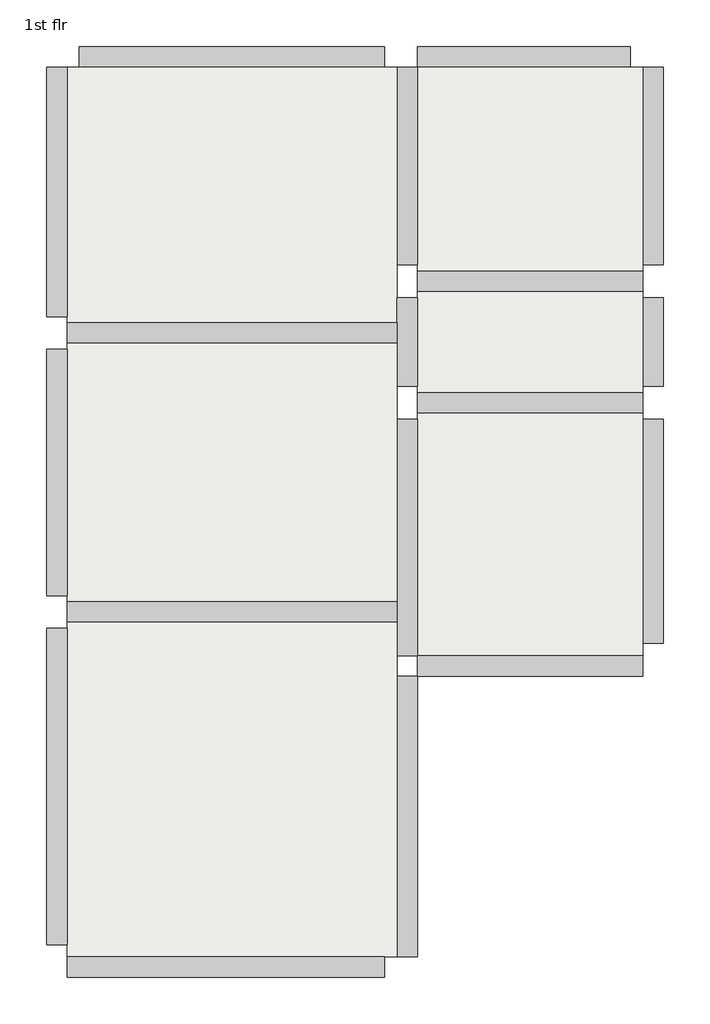
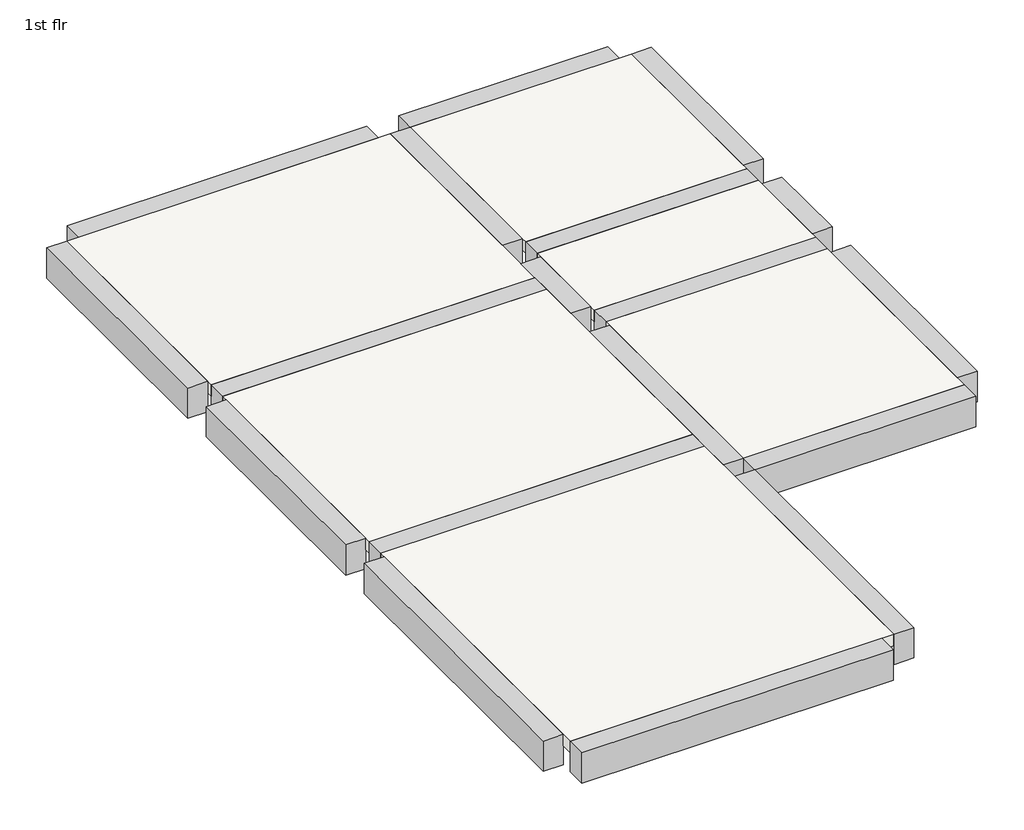
# One storey, part 1 of 2: 18 beams, 6 slabs.
"""IFC4 building model written with IfcOpenShell, lengths in millimetres."""

from ifc_helpers import new_model, si_unit, frame, origin, place, context, project, spatial, polyline, outline, extrude, faceted_brep, element, save

model = new_model("IFC4")

# Units and contexts
model_context = context("Model", 3, world=origin())
ifc_project = project(units=[si_unit("LENGTHUNIT", "METRE", prefix="MILLI")], contexts=[model_context])

# Site, building, storey
site = spatial("IfcSite", under=ifc_project)
building = spatial("IfcBuilding", under=site)
storey = spatial("IfcBuildingStorey", under=building, Name="1st flr", Elevation=3200.4)

# Beams
placement = place(None, origin())
element("IfcBeam", 1, ObjectType="Concrete-Rectangular Beam : BEAM", at=placement, inside=storey, context=model_context, shape_type="SweptSolid", body=[
    extrude(outline(polyline([(-12336.5990423, 3901.2699494), (-12082.5990423, 3901.2699494), (-12082.5990423, -16.6800506), (-12336.5990423, -16.6800506), (-12336.5990423, 3901.2699494)])), frame((0.0, 0.0, 2794.0), z_axis=(0.0, 0.0, 1.0), x_axis=(1.0, 0.0, 0.0)), (0.0, 0.0, 1.0), 406.4),
])
element("IfcBeam", 2, ObjectType="Concrete-Rectangular Beam : BEAM", at=placement, inside=storey, context=model_context, shape_type="SweptSolid", body=[
    extrude(outline(polyline([(-12336.5990423, 7355.6699494), (-12082.5990423, 7355.6699494), (-12082.5990423, 4307.6699494), (-12336.5990423, 4307.6699494), (-12336.5990423, 7355.6699494)])), frame((0.0, 0.0, 2794.0), z_axis=(0.0, 0.0, 1.0), x_axis=(1.0, 0.0, 0.0)), (0.0, 0.0, 1.0), 406.4),
])
element("IfcBeam", 3, ObjectType="Concrete-Rectangular Beam : BEAM", at=placement, inside=storey, context=model_context, shape_type="Brep", body=[
    faceted_brep([(-12082.5990423, 10854.5199494, 3200.4), (-12336.5990423, 10854.5199494, 3200.4), (-12336.5990423, 7762.0699494, 3200.4), (-12082.5990423, 7762.0699494, 3200.4), (-12082.5990423, 10854.5199494, 2794.0), (-12082.5990423, 10854.5199494, 3048.0), (-12082.5990423, 7762.0699494, 2794.0), (-12336.5990423, 10854.5199494, 2794.0), (-12336.5990423, 7762.0699494, 2794.0)], [[[0, 1, 2, 3]], [[4, 5, 0, 3, 6]], [[7, 4, 6, 8]], [[1, 7, 8, 2]], [[1, 0, 5, 4, 7]], [[3, 2, 8, 6]]]),
])
element("IfcBeam", 4, ObjectType="Concrete-Rectangular Beam : BEAM", at=placement, inside=storey, context=model_context, shape_type="SweptSolid", body=[
    extrude(outline(polyline([(-11930.1990423, 10854.5199494), (-11930.1990423, 11108.5199494), (-8145.5990423, 11108.5199494), (-8145.5990423, 10854.5199494), (-11930.1990423, 10854.5199494)])), frame((0.0, 0.0, 2794.0), z_axis=(0.0, 0.0, 1.0), x_axis=(1.0, 0.0, 0.0)), (0.0, 0.0, 1.0), 406.4),
])
element("IfcBeam", 5, ObjectType="Concrete-Rectangular Beam : BEAM", at=placement, inside=storey, context=model_context, shape_type="Brep", body=[
    faceted_brep([(-7739.1990423, 11108.5199494, 3200.4), (-7739.1990423, 10854.5199494, 3200.4), (-5097.5990423, 10854.5199494, 3200.4), (-5097.5990423, 11108.5199494, 3200.4), (-7739.1990423, 10854.5199494, 3048.0), (-7739.1990423, 10854.5199494, 2794.0), (-5097.5990423, 10854.5199494, 2794.0), (-7739.1990423, 11108.5199494, 2794.0), (-5097.5990423, 11108.5199494, 2794.0)], [[[0, 1, 2, 3]], [[1, 4, 5, 6, 2]], [[5, 7, 8, 6]], [[7, 0, 3, 8]], [[5, 4, 1, 0, 7]], [[3, 2, 6, 8]]]),
])
element("IfcBeam", 6, ObjectType="Concrete-Rectangular Beam : BEAM", at=placement, inside=storey, context=model_context, shape_type="Brep", body=[
    faceted_brep([(-4691.1990423, 10854.5199494, 3200.4), (-4945.1990423, 10854.5199494, 3200.4), (-4945.1990423, 8403.4199494, 3200.4), (-4691.1990423, 8403.4199494, 3200.4), (-4691.1990423, 10854.5199494, 2794.0), (-4691.1990423, 8403.4199494, 2794.0), (-4945.1990423, 10854.5199494, 2794.0), (-4945.1990423, 8403.4199494, 2794.0), (-4945.1990423, 10854.5199494, 3048.0)], [[[0, 1, 2, 3]], [[4, 0, 3, 5]], [[6, 4, 5, 7]], [[1, 8, 6, 7, 2]], [[6, 8, 1, 0, 4]], [[3, 2, 7, 5]]]),
])
element("IfcBeam", 7, ObjectType="Concrete-Rectangular Beam : BEAM", at=placement, inside=storey, context=model_context, shape_type="SweptSolid", body=[
    extrude(outline(polyline([(-4945.1990423, 7997.0199494), (-4691.1990423, 7997.0199494), (-4691.1990423, 6898.4699494), (-4945.1990423, 6898.4699494), (-4945.1990423, 7997.0199494)])), frame((0.0, 0.0, 2794.0), z_axis=(0.0, 0.0, 1.0), x_axis=(1.0, 0.0, 0.0)), (0.0, 0.0, 1.0), 406.4),
])
element("IfcBeam", 8, ObjectType="Concrete-Rectangular Beam : BEAM", at=placement, inside=storey, context=model_context, shape_type="SweptSolid", body=[
    extrude(outline(polyline([(-4691.1990423, 3717.1199494), (-4945.1990423, 3717.1199494), (-4945.1990423, 6492.0699494), (-4691.1990423, 6492.0699494), (-4691.1990423, 3717.1199494)])), frame((0.0, 0.0, 2794.0), z_axis=(0.0, 0.0, 1.0), x_axis=(1.0, 0.0, 0.0)), (0.0, 0.0, 1.0), 406.4),
])
element("IfcBeam", 9, ObjectType="Concrete-Rectangular Beam : BEAM", at=placement, inside=storey, context=model_context, shape_type="Brep", body=[
    faceted_brep([(-4945.1990423, 3310.7199494, 3200.4), (-4945.1990423, 3564.7199494, 3200.4), (-7739.1990423, 3564.7199494, 3200.4), (-7739.1990423, 3310.7199494, 3200.4), (-4945.1990423, 3564.7199494, 3048.0), (-4945.1990423, 3564.7199494, 2794.0), (-7739.1990423, 3564.7199494, 2794.0), (-7739.1990423, 3564.7199494, 3048.0), (-4945.1990423, 3310.7199494, 2794.0), (-7739.1990423, 3310.7199494, 2794.0)], [[[0, 1, 2, 3]], [[1, 4, 5, 6, 7, 2]], [[5, 8, 9, 6]], [[3, 9, 8, 0]], [[0, 8, 5, 4, 1]], [[3, 2, 7, 6, 9]]]),
])
element("IfcBeam", 10, ObjectType="Concrete-Rectangular Beam : BEAM", at=placement, inside=storey, context=model_context, shape_type="Brep", body=[
    faceted_brep([(-7993.1990423, 3564.7199494, 3200.4), (-7739.1990423, 3564.7199494, 3200.4), (-7739.1990423, 6492.0699494, 3200.4), (-7993.1990423, 6492.0699494, 3200.4), (-7993.1990423, 4231.4699494, 3200.4), (-7993.1990423, 3977.4699494, 3200.4), (-7993.1990423, 3564.7199494, 2794.0), (-7993.1990423, 6492.0699494, 2794.0), (-7993.1990423, 4231.4699494, 2794.0), (-7993.1990423, 3977.4699494, 2794.0), (-7739.1990423, 3564.7199494, 2794.0), (-7739.1990423, 6492.0699494, 2794.0), (-7739.1990423, 3564.7199494, 3048.0)], [[[0, 1, 2, 3, 4, 5]], [[6, 0, 5, 4, 3, 7, 8, 9]], [[10, 6, 9, 8, 7, 11]], [[1, 12, 10, 11, 2]], [[10, 12, 1, 0, 6]], [[3, 2, 11, 7]]]),
])
element("IfcBeam", 11, ObjectType="Concrete-Rectangular Beam : BEAM", at=placement, inside=storey, context=model_context, shape_type="Brep", body=[
    faceted_brep([(-7993.1990423, 6898.4699494, 3200.4), (-7739.1990423, 6898.4699494, 3200.4), (-7739.1990423, 7997.0199494, 3200.4), (-7993.1990423, 7997.0199494, 3200.4), (-7993.1990423, 7685.8699494, 3200.4), (-7993.1990423, 7431.8699494, 3200.4), (-7739.1990423, 6898.4699494, 2794.0), (-7739.1990423, 7997.0199494, 2794.0), (-7993.1990423, 6898.4699494, 2794.0), (-7993.1990423, 7431.8699494, 2794.0), (-7993.1990423, 7685.8699494, 2794.0), (-7993.1990423, 7997.0199494, 2794.0)], [[[0, 1, 2, 3, 4, 5]], [[1, 6, 7, 2]], [[6, 8, 9, 10, 11, 7]], [[8, 0, 5, 4, 3, 11, 10, 9]], [[1, 0, 8, 6]], [[3, 2, 7, 11]]]),
])
element("IfcBeam", 12, ObjectType="Concrete-Rectangular Beam : BEAM", at=placement, inside=storey, context=model_context, shape_type="Brep", body=[
    faceted_brep([(-7739.1990423, 10854.5199494, 3200.4), (-7993.1990423, 10854.5199494, 3200.4), (-7993.1990423, 8403.4199494, 3200.4), (-7739.1990423, 8403.4199494, 3200.4), (-7739.1990423, 10854.5199494, 2794.0), (-7739.1990423, 10854.5199494, 3048.0), (-7739.1990423, 8403.4199494, 2794.0), (-7993.1990423, 10854.5199494, 2794.0), (-7993.1990423, 8403.4199494, 2794.0), (-7993.1990423, 10854.5199494, 3048.0)], [[[0, 1, 2, 3]], [[4, 5, 0, 3, 6]], [[7, 4, 6, 8]], [[1, 9, 7, 8, 2]], [[7, 9, 1, 0, 5, 4]], [[3, 2, 8, 6]]]),
])
element("IfcBeam", 13, ObjectType="Concrete-Rectangular Beam : BEAM", at=placement, inside=storey, context=model_context, shape_type="Brep", body=[
    faceted_brep([(-7739.1990423, 3310.7199494, 3200.4), (-7993.1990423, 3310.7199494, 3200.4), (-7993.1990423, -169.0800506, 3200.4), (-7739.1990423, -169.0800506, 3200.4), (-7993.1990423, 3310.7199494, 2794.0), (-7993.1990423, -169.0800506, 2794.0), (-7993.1990423, -169.0800506, 3048.0), (-7739.1990423, 3310.7199494, 2794.0), (-7739.1990423, -169.0800506, 2794.0)], [[[0, 1, 2, 3]], [[1, 4, 5, 6, 2]], [[4, 7, 8, 5]], [[7, 0, 3, 8]], [[0, 7, 4, 1]], [[3, 2, 6, 5, 8]]]),
])
element("IfcBeam", 14, ObjectType="Concrete-Rectangular Beam : BEAM", at=placement, inside=storey, context=model_context, shape_type="Brep", body=[
    faceted_brep([(-12082.5990423, -169.0800506, 3200.4), (-12082.5990423, -423.0800506, 3200.4), (-8145.5990423, -423.0800506, 3200.4), (-8145.5990423, -169.0800506, 3200.4), (-12082.5990423, -169.0800506, 2794.0), (-12082.5990423, -169.0800506, 3048.0), (-8145.5990423, -169.0800506, 2794.0), (-12082.5990423, -423.0800506, 2794.0), (-8145.5990423, -423.0800506, 2794.0)], [[[0, 1, 2, 3]], [[4, 5, 0, 3, 6]], [[7, 4, 6, 8]], [[1, 7, 8, 2]], [[0, 5, 4, 7, 1]], [[3, 2, 8, 6]]]),
])
element("IfcBeam", 15, ObjectType="Concrete-Rectangular Beam : BEAM", at=placement, inside=storey, context=model_context, shape_type="Brep", body=[
    faceted_brep([(-12082.5990423, 7685.8699494, 3200.4), (-12082.5990423, 7431.8699494, 3200.4), (-7993.1990423, 7431.8699494, 3200.4), (-7993.1990423, 7685.8699494, 3200.4), (-12082.5990423, 7431.8699494, 3048.0), (-12082.5990423, 7431.8699494, 2794.0), (-7993.1990423, 7431.8699494, 2794.0), (-7993.1990423, 7431.8699494, 3048.0), (-12082.5990423, 7685.8699494, 2794.0), (-7993.1990423, 7685.8699494, 2794.0), (-7993.1990423, 7685.8699494, 3048.0), (-12082.5990423, 7685.8699494, 3048.0)], [[[0, 1, 2, 3]], [[1, 4, 5, 6, 7, 2]], [[5, 8, 9, 6]], [[3, 10, 9, 8, 11, 0]], [[0, 11, 8, 5, 4, 1]], [[3, 2, 7, 6, 9, 10]]]),
])
element("IfcBeam", 16, ObjectType="Concrete-Rectangular Beam : BEAM", at=placement, inside=storey, context=model_context, shape_type="Brep", body=[
    faceted_brep([(-7739.1990423, 8327.2199494, 3200.4), (-7739.1990423, 8073.2199494, 3200.4), (-4945.1990423, 8073.2199494, 3200.4), (-4945.1990423, 8327.2199494, 3200.4), (-7739.1990423, 8073.2199494, 3048.0), (-7739.1990423, 8073.2199494, 2794.0), (-4945.1990423, 8073.2199494, 2794.0), (-4945.1990423, 8073.2199494, 3048.0), (-7739.1990423, 8327.2199494, 2794.0), (-4945.1990423, 8327.2199494, 2794.0), (-4945.1990423, 8327.2199494, 3048.0), (-7739.1990423, 8327.2199494, 3048.0)], [[[0, 1, 2, 3]], [[1, 4, 5, 6, 7, 2]], [[5, 8, 9, 6]], [[3, 10, 9, 8, 11, 0]], [[9, 10, 3, 2, 7, 6]], [[0, 11, 8, 5, 4, 1]]]),
])
element("IfcBeam", 17, ObjectType="Concrete-Rectangular Beam : BEAM", at=placement, inside=storey, context=model_context, shape_type="Brep", body=[
    faceted_brep([(-4945.1990423, 6568.2699494, 3200.4), (-4945.1990423, 6822.2699494, 3200.4), (-7739.1990423, 6822.2699494, 3200.4), (-7739.1990423, 6568.2699494, 3200.4), (-7739.1990423, 6568.2699494, 3048.0), (-7739.1990423, 6568.2699494, 2794.0), (-4945.1990423, 6568.2699494, 2794.0), (-4945.1990423, 6568.2699494, 3048.0), (-4945.1990423, 6822.2699494, 2794.0), (-7739.1990423, 6822.2699494, 2794.0), (-4945.1990423, 6822.2699494, 3048.0), (-7739.1990423, 6822.2699494, 3048.0)], [[[0, 1, 2, 3]], [[3, 4, 5, 6, 7, 0]], [[8, 6, 5, 9]], [[1, 10, 8, 9, 11, 2]], [[5, 4, 3, 2, 11, 9]], [[0, 7, 6, 8, 10, 1]]]),
])
element("IfcBeam", 18, ObjectType="Concrete-Rectangular Beam : BEAM", at=placement, inside=storey, context=model_context, shape_type="Brep", body=[
    faceted_brep([(-12082.5990423, 4231.4699494, 3200.4), (-12082.5990423, 3977.4699494, 3200.4), (-7993.1990423, 3977.4699494, 3200.4), (-7993.1990423, 4231.4699494, 3200.4), (-12082.5990423, 3977.4699494, 3048.0), (-12082.5990423, 3977.4699494, 2794.0), (-7993.1990423, 3977.4699494, 2794.0), (-7993.1990423, 3977.4699494, 3048.0), (-12082.5990423, 4231.4699494, 2794.0), (-7993.1990423, 4231.4699494, 2794.0), (-7993.1990423, 4231.4699494, 3048.0), (-12082.5990423, 4231.4699494, 3048.0)], [[[0, 1, 2, 3]], [[1, 4, 5, 6, 7, 2]], [[5, 8, 9, 6]], [[3, 10, 9, 8, 11, 0]], [[0, 11, 8, 5, 4, 1]], [[3, 2, 7, 6, 9, 10]]]),
])

# Slabs
element("IfcSlab", 19, ObjectType="6\" Foundation Slab", at=placement, inside=storey, context=model_context, shape_type="Brep", body=[
    faceted_brep([(-7993.1990423, 10854.5199494, 3048.0), (-7993.1990423, 7685.8699494, 3048.0), (-12082.5990423, 7685.8699494, 3048.0), (-12082.5990423, 10854.5199494, 3048.0), (-7993.1990423, 10854.5199494, 3200.4), (-8145.5990423, 10854.5199494, 3200.4), (-11930.1990423, 10854.5199494, 3200.4), (-12082.5990423, 10854.5199494, 3200.4), (-12082.5990423, 7762.0699494, 3200.4), (-12082.5990423, 7685.8699494, 3200.4), (-7993.1990423, 7685.8699494, 3200.4), (-7993.1990423, 7997.0199494, 3200.4), (-7993.1990423, 8403.4199494, 3200.4)], [[[0, 1, 2, 3]], [[4, 5, 6, 7, 8, 9, 10, 11, 12]], [[1, 0, 4, 12, 11, 10]], [[2, 1, 10, 9]], [[3, 2, 9, 8, 7]], [[0, 3, 7, 6, 5, 4]]]),
])
element("IfcSlab", 20, ObjectType="6\" Foundation Slab", at=placement, inside=storey, context=model_context, shape_type="Brep", body=[
    faceted_brep([(-4945.1990423, 10854.5199494, 3048.0), (-4945.1990423, 8327.2199494, 3048.0), (-7739.1990423, 8327.2199494, 3048.0), (-7739.1990423, 10854.5199494, 3048.0), (-4945.1990423, 10854.5199494, 3200.4), (-5097.5990423, 10854.5199494, 3200.4), (-7739.1990423, 10854.5199494, 3200.4), (-7739.1990423, 8403.4199494, 3200.4), (-7739.1990423, 8327.2199494, 3200.4), (-4945.1990423, 8327.2199494, 3200.4), (-4945.1990423, 8403.4199494, 3200.4)], [[[0, 1, 2, 3]], [[4, 5, 6, 7, 8, 9, 10]], [[1, 0, 4, 10, 9]], [[2, 1, 9, 8]], [[3, 2, 8, 7, 6]], [[0, 3, 6, 5, 4]]]),
])
element("IfcSlab", 21, ObjectType="6\" Foundation Slab", at=placement, inside=storey, context=model_context, shape_type="Brep", body=[
    faceted_brep([(-7993.1990423, 7431.8699494, 3048.0), (-7993.1990423, 4231.4699494, 3048.0), (-12082.5990423, 4231.4699494, 3048.0), (-12082.5990423, 7431.8699494, 3048.0), (-7993.1990423, 7431.8699494, 3200.4), (-12082.5990423, 7431.8699494, 3200.4), (-12082.5990423, 7355.6699494, 3200.4), (-12082.5990423, 4307.6699494, 3200.4), (-12082.5990423, 4231.4699494, 3200.4), (-7993.1990423, 4231.4699494, 3200.4), (-7993.1990423, 6492.0699494, 3200.4), (-7993.1990423, 6898.4699494, 3200.4)], [[[0, 1, 2, 3]], [[4, 5, 6, 7, 8, 9, 10, 11]], [[1, 0, 4, 11, 10, 9]], [[2, 1, 9, 8]], [[3, 2, 8, 7, 6, 5]], [[0, 3, 5, 4]]]),
])
element("IfcSlab", 22, ObjectType="6\" Foundation Slab", at=placement, inside=storey, context=model_context, shape_type="Brep", body=[
    faceted_brep([(-4945.1990423, 6568.2699494, 3048.0), (-4945.1990423, 3564.7199494, 3048.0), (-7739.1990423, 3564.7199494, 3048.0), (-7739.1990423, 6568.2699494, 3048.0), (-4945.1990423, 6568.2699494, 3200.4), (-7739.1990423, 6568.2699494, 3200.4), (-7739.1990423, 6492.0699494, 3200.4), (-7739.1990423, 3564.7199494, 3200.4), (-4945.1990423, 3564.7199494, 3200.4), (-4945.1990423, 3717.1199494, 3200.4), (-4945.1990423, 6492.0699494, 3200.4)], [[[0, 1, 2, 3]], [[4, 5, 6, 7, 8, 9, 10]], [[1, 0, 4, 10, 9, 8]], [[2, 1, 8, 7]], [[3, 2, 7, 6, 5]], [[0, 3, 5, 4]]]),
])
element("IfcSlab", 23, ObjectType="6\" Foundation Slab", at=placement, inside=storey, context=model_context, shape_type="Brep", body=[
    faceted_brep([(-7993.1990423, 3977.4699494, 3048.0), (-7993.1990423, -169.0800506, 3048.0), (-12082.5990423, -169.0800506, 3048.0), (-12082.5990423, 3977.4699494, 3048.0), (-7993.1990423, 3977.4699494, 3200.4), (-12082.5990423, 3977.4699494, 3200.4), (-12082.5990423, 3901.2699494, 3200.4), (-12082.5990423, -16.6800506, 3200.4), (-12082.5990423, -169.0800506, 3200.4), (-8145.5990423, -169.0800506, 3200.4), (-7993.1990423, -169.0800506, 3200.4), (-7993.1990423, 3310.7199494, 3200.4), (-7993.1990423, 3564.7199494, 3200.4)], [[[0, 1, 2, 3]], [[4, 5, 6, 7, 8, 9, 10, 11, 12]], [[1, 0, 4, 12, 11, 10]], [[2, 1, 10, 9, 8]], [[3, 2, 8, 7, 6, 5]], [[0, 3, 5, 4]]]),
])
element("IfcSlab", 24, ObjectType="6\" Foundation Slab", at=placement, inside=storey, context=model_context, shape_type="Brep", body=[
    faceted_brep([(-4945.1990423, 8073.2199494, 3048.0), (-4945.1990423, 6822.2699494, 3048.0), (-7739.1990423, 6822.2699494, 3048.0), (-7739.1990423, 8073.2199494, 3048.0), (-4945.1990423, 8073.2199494, 3200.4), (-7739.1990423, 8073.2199494, 3200.4), (-7739.1990423, 7997.0199494, 3200.4), (-7739.1990423, 6898.4699494, 3200.4), (-7739.1990423, 6822.2699494, 3200.4), (-4945.1990423, 6822.2699494, 3200.4), (-4945.1990423, 6898.4699494, 3200.4), (-4945.1990423, 7997.0199494, 3200.4)], [[[0, 1, 2, 3]], [[4, 5, 6, 7, 8, 9, 10, 11]], [[1, 0, 4, 11, 10, 9]], [[2, 1, 9, 8]], [[3, 2, 8, 7, 6, 5]], [[0, 3, 5, 4]]]),
])

save(model, "model.ifc")

# Revit data of these elements
# Type "Concrete-Rectangular Beam : BEAM"
#   Assembly Code = "B10"
#   Length [instance default] = 1524 mm
#   b = 254 mm
#   h = 406.4 mm
#   Structural Material [instance default] = Concrete, Cast-in-Place gray
# Type "6\" Foundation Slab"
#   Layers, outside or top first: 152.4 mm "Concrete, Cast-in-Place gray" (function 1)
# Elements 1, 2, 3, 4, 5, 6, 7, 8, 9, 10, 11, 12, 13, 14, 15, 16, 17, 18 (IfcBeam, "Concrete-Rectangular Beam : BEAM")
#   Structural Material = Concrete, Cast-in-Place gray
#   Phase Created = New Construction
#   Materials on its faces: "Concrete, Cast-in-Place gray"
# Elements 19, 20, 21, 22, 23, 24 (IfcSlab, "6\" Foundation Slab")
#   Height Offset From Level = 0 mm
#   built-in parameter 1001954 = 1
#   Phase Created = New Construction
#   Materials on its faces: "Concrete, Cast-in-Place gray"
# Materials
#   "Concrete, Cast-in-Place gray": class "Concrete", colour RGB 192 192 192, transparency 0, Description = "Cast-in-place concrete", Cost = 0
